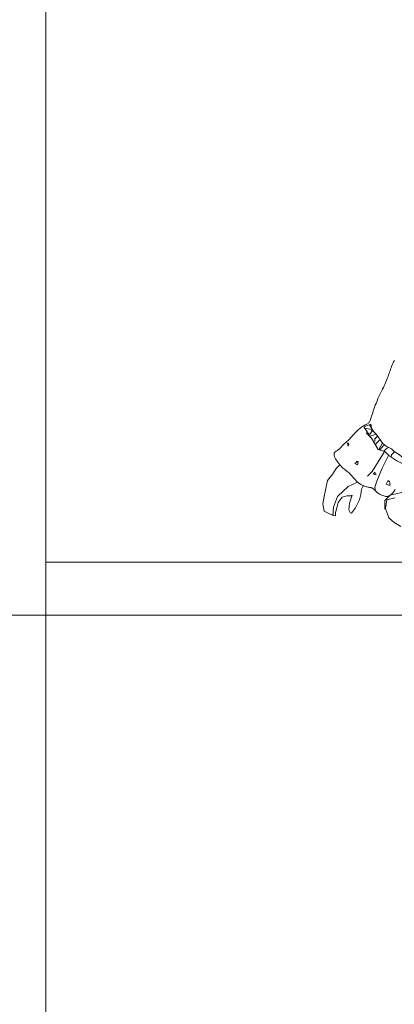
# Model space of a CAD drawing. Units: inches. Extents: x -17 to 1735, y -531 to 60.
# Tile 19 of 27: x 1734.79189 to 1734.79885, y -150.22283 to -150.20455. Entities that reach past the tile are written whole.
import ezdxf

# ---------------------------------------------------------------- set-up
doc = ezdxf.new("R2010")
doc.units = ezdxf.units.IN
doc.header["$MEASUREMENT"] = 0
doc.layers.add('A-FURN', color=242, linetype='Continuous', lineweight=18, true_color=0xcd2027)

# ---------------------------------------------------------------- blocks, each defined once
blk = doc.blocks.new('childrens_room_2')
for p, q in [((73.14631, 53.98246), (73.14631, 54.72383)), ((73.63163, 54.20212), (73.14631, 54.20212)), ((73.86245, 54.17714), (73.12162, 54.17714))]:
    blk.add_line(p, q)
for points in [[(73.31069, 54.29728), (73.31032, 54.29655), (73.30998, 54.29583), (73.30966, 54.29513), (73.30937, 54.29443), (73.30911, 54.29375), (73.30886, 54.29308), (73.30864, 54.29241), (73.30842, 54.29174), (73.3082, 54.29107), (73.30798, 54.29039), (73.30774, 54.28969), (73.30748, 54.28897), (73.30719, 54.28823), (73.30687, 54.28748), (73.30654, 54.28671), (73.30619, 54.28595), (73.30584, 54.28519), (73.30549, 54.28445), (73.30514, 54.28373), (73.3048, 54.28304), (73.30447, 54.28239), (73.30415, 54.28176), (73.30384, 54.28115), (73.30354, 54.28054), (73.30324, 54.27991), (73.30294, 54.27925), (73.30264, 54.27855), (73.30233, 54.27779), (73.30201, 54.27697), (73.30168, 54.27611), (73.30136, 54.27521), (73.30104, 54.27431), (73.30074, 54.27342), (73.30046, 54.27256), (73.30019, 54.27175), (73.29996, 54.27102), (73.29976, 54.27038), (73.29958, 54.26982), (73.29942, 54.26934), (73.29927, 54.26892), (73.29912, 54.26857), (73.29895, 54.26826), (73.29876, 54.268), (73.29854, 54.26777), (73.29829, 54.26756), (73.29799, 54.26737), (73.29767, 54.26719), (73.29731, 54.26701), (73.29693, 54.26681), (73.29652, 54.2666), (73.2961, 54.26636), (73.29565, 54.26609), (73.29519, 54.26577), (73.29472, 54.26542), (73.29425, 54.26504), (73.29378, 54.26463), (73.29332, 54.26421), (73.29287, 54.26379), (73.29243, 54.26336), (73.29203, 54.26294), (73.29165, 54.26253), (73.29129, 54.26214), (73.29095, 54.26176), (73.29063, 54.26139), (73.29031, 54.26103), (73.28999, 54.26068), (73.28967, 54.26034), (73.28935, 54.26), (73.289, 54.25967), (73.28865, 54.25934), (73.28829, 54.25902), (73.28793, 54.2587), (73.28758, 54.25838), (73.28723, 54.25806), (73.28689, 54.25774), (73.28656, 54.25743), (73.28625, 54.25711), (73.28596, 54.2568), (73.28569, 54.2565), (73.28542, 54.2562), (73.28515, 54.25592), (73.28489, 54.25565), (73.28463, 54.2554), (73.28435, 54.25517), (73.28407, 54.25497), (73.28379, 54.25478), (73.28351, 54.25461), (73.28324, 54.25444), (73.28299, 54.25427), (73.28276, 54.25409), (73.28257, 54.25391), (73.28241, 54.2537), (73.28229, 54.25347), (73.28223, 54.25322), (73.28221, 54.25293), (73.28224, 54.25261), (73.28233, 54.25225), (73.28247, 54.25185), (73.28267, 54.25141), (73.28293, 54.25092), (73.28326, 54.25039), (73.28364, 54.24982), (73.28406, 54.24923), (73.28451, 54.24864), (73.28498, 54.24806), (73.28546, 54.2475), (73.28594, 54.24698), (73.2864, 54.24651), (73.28685, 54.24611), (73.28727, 54.24576), (73.28768, 54.24545), (73.28808, 54.24515), (73.28848, 54.24485), (73.28888, 54.24453), (73.28929, 54.24418), (73.28971, 54.24378), (73.29016, 54.24332), (73.29062, 54.2428), (73.2911, 54.24225), (73.2916, 54.24168), (73.29211, 54.2411), (73.29265, 54.24054), (73.2932, 54.24001), (73.29376, 54.23953), (73.29434, 54.23911), (73.29492, 54.23875), (73.29551, 54.23844), (73.29608, 54.23818), (73.29664, 54.23797), (73.29717, 54.23779), (73.29766, 54.23765), (73.29812, 54.23754), (73.29853, 54.23745), (73.2989, 54.23738), (73.29923, 54.23732), (73.29953, 54.23726), (73.2998, 54.23719), (73.30006, 54.2371), (73.3003, 54.23699), (73.30054, 54.23686), (73.30078, 54.23668), (73.30102, 54.23647), (73.30127, 54.23623), (73.30152, 54.23598), (73.3018, 54.2357), (73.30209, 54.23542), (73.30241, 54.23514), (73.30275, 54.23486), (73.30311, 54.23459), (73.30351, 54.23433), (73.30392, 54.23409), (73.30435, 54.23387), (73.30479, 54.23367), (73.30523, 54.2335), (73.30567, 54.23335), (73.30611, 54.23323), (73.30654, 54.23315), (73.30696, 54.23312), (73.30738, 54.23314), (73.3078, 54.23323), (73.30823, 54.23339), (73.30867, 54.23364), (73.30911, 54.23399), (73.30958, 54.23444), (73.31006, 54.23501), (73.31055, 54.23567), (73.31104, 54.23641)], [(73.30021, 54.26473), (73.3002, 54.26369), (73.29957, 54.26716), (73.29641, 54.2659), (73.29641, 54.26558), (73.29862, 54.26243), (73.29736, 54.26306), (73.29988, 54.26054), (73.30303, 54.25519), (73.30619, 54.25425), (73.30808, 54.25236), (73.31186, 54.24984), (73.31565, 54.24795), (73.31785, 54.24795)], [(73.29988, 54.26464), (73.29673, 54.26527)], [(73.29894, 54.26684), (73.30083, 54.26369), (73.30209, 54.26243), (73.30303, 54.26117), (73.30524, 54.25803), (73.30682, 54.25677), (73.30934, 54.25551), (73.3106, 54.25425), (73.31312, 54.25267), (73.31533, 54.25078), (73.31754, 54.24826)], [(73.3002, 54.26401), (73.29894, 54.26212)], [(73.30209, 54.26243), (73.29925, 54.26149)], [(73.30272, 54.26149), (73.30146, 54.26023), (73.30146, 54.25897)], [(73.31093, 54.2325), (73.30715, 54.23155), (73.30652, 54.22746), (73.30809, 54.22305), (73.31062, 54.22085), (73.31377, 54.21896)], [(73.28853, 54.25803), (73.28885, 54.25677), (73.28916, 54.25771), (73.28853, 54.25834)], [(73.30367, 54.2596), (73.30209, 54.25803), (73.30177, 54.25708)], [(73.30493, 54.25803), (73.30367, 54.25582), (73.30367, 54.25519)], [(73.30619, 54.2574), (73.30524, 54.25677), (73.30398, 54.25519)], [(73.30776, 54.25614), (73.30682, 54.25551), (73.30587, 54.25456)], [(73.30587, 54.25393), (73.3002, 54.2448), (73.29799, 54.2426)], [(73.30808, 54.25267), (73.30493, 54.24637), (73.3024, 54.24039), (73.30146, 54.23756), (73.30177, 54.23567)], [(73.3106, 54.25393), (73.30934, 54.25267), (73.30934, 54.25204)], [(73.28476, 54.24793), (73.28318, 54.24635), (73.28161, 54.24383), (73.27909, 54.24069), (73.27751, 54.23313), (73.27688, 54.22966), (73.27751, 54.2262), (73.28003, 54.22494), (73.28287, 54.224), (73.28287, 54.22557), (73.2835, 54.22777), (73.28413, 54.23029), (73.28602, 54.23281), (73.28823, 54.23344), (73.29044, 54.23344), (73.29075, 54.23376), (73.28949, 54.22998), (73.28918, 54.22683), (73.28981, 54.22557), (73.29044, 54.22525), (73.29138, 54.22651), (73.29233, 54.22777), (73.29422, 54.23155), (73.29485, 54.23407), (73.29517, 54.23659), (73.29611, 54.23848)], [(73.29295, 54.24921), (73.292, 54.24858), (73.29326, 54.24795), (73.29358, 54.24952), (73.29263, 54.24952)], [(73.30146, 54.24448), (73.30083, 54.24354), (73.30209, 54.24323), (73.30146, 54.24448)], [(73.29296, 54.23974), (73.28886, 54.23785), (73.28382, 54.23313), (73.28192, 54.22809), (73.28161, 54.224)], [(73.30776, 54.24071), (73.30682, 54.23882), (73.30808, 54.2385), (73.30871, 54.2385), (73.30839, 54.24039), (73.30745, 54.24039)], [(73.31976, 54.23628), (73.31408, 54.23502), (73.30872, 54.23376), (73.3062, 54.23124), (73.3062, 54.22714)]]:
    blk.add_lwpolyline(points)

msp = doc.modelspace()

# ---------------------------------------------------------------- block references
at = {"layer": 'A-FURN', "xscale": 0.0393700787401575, "yscale": 0.0393700787401575, "zscale": 0.0393700787401575}
msp.add_blockref('childrens_room_2', (1731.912601, -152.348565), dxfattribs=at)

doc.saveas('drawing.dxf')
